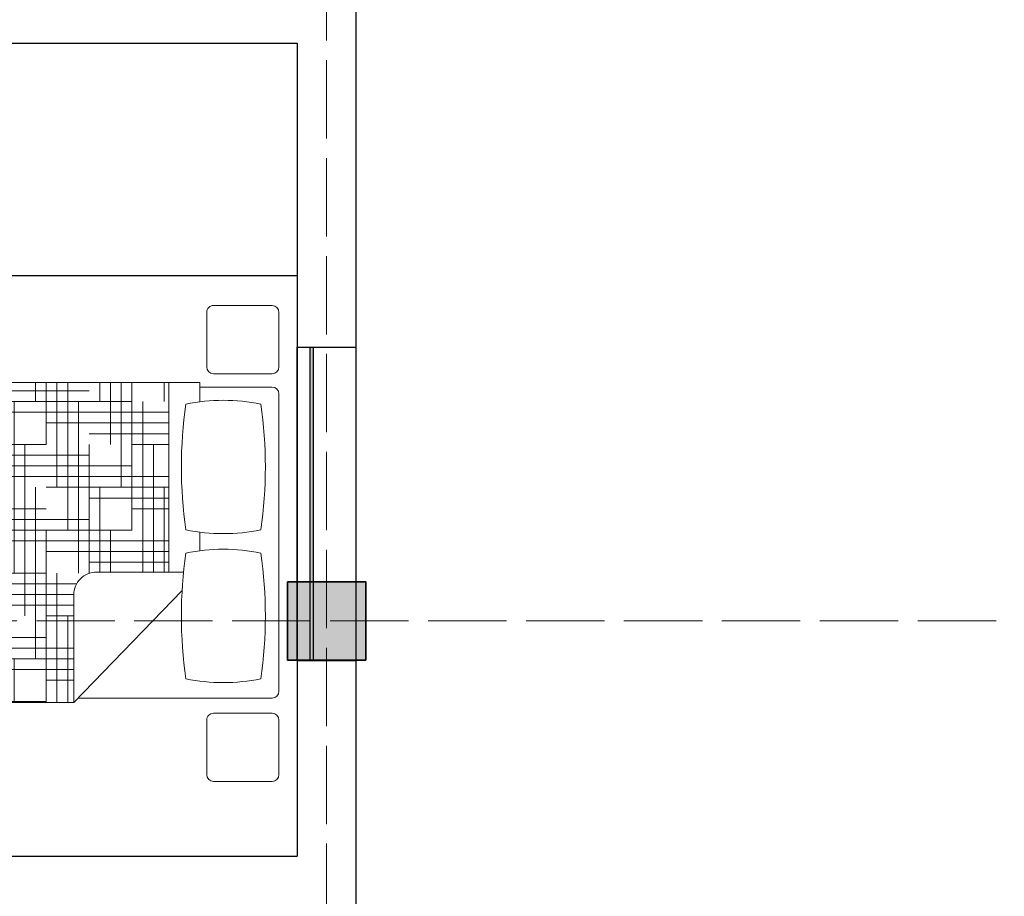
# Model space of a CAD drawing. Units: inches. Extents: x -113 to 5399, y -1393 to 3302.
# Tile 39 of 40: x 3612 to 3763, y 2903 to 3038. Entities that reach past the tile are written whole.
import ezdxf

# ---------------------------------------------------------------- set-up
doc = ezdxf.new("R2010")
doc.units = ezdxf.units.IN
doc.header["$MEASUREMENT"] = 0
doc.linetypes.add('ACAD_ISO02W100', pattern=[15, 12, -3])
for name, color, linetype, lineweight in [('A-ANNO-DIMS', 254, 'Continuous', 18), ('A-COLS', 7, 'Continuous', 35), ('furniture', 131, 'Continuous', 18), ('GRIDS', 7, 'ACAD_ISO02W100', 13), ('walls', 1, 'Continuous', 25), ('windows', 3, 'Continuous', 25)]:
    doc.layers.add(name, color=color, linetype=linetype, lineweight=lineweight)
doc.styles.get("Standard").update_dxf_attribs({"font": 'arial.ttf'})
doc.dimstyles.get("Standard").update_dxf_attribs({"dimtxt": 6, "dimasz": 0.18, "dimexe": 0.18, "dimexo": 0.0625, "dimgap": 0.09, "dimtad": 0, "dimtih": 1, "dimtoh": 1, "dimdec": 1, "dimzin": 0, "dimdsep": 46, "dimlunit": 4, "dimtxsty": 'Standard', "dimblk": 'ARCHTICK', "dimcen": 0.09, "dimadec": 0, "dimazin": 0, "dimtfac": 1, "dimtdec": 1, "dimtofl": 0, "dimtmove": 0, "dimatfit": 3, "dimfxl": 1, "dimtolj": 1, "dimtzin": 0, "dimarcsym": 0})

# ---------------------------------------------------------------- blocks, each defined once
blk = doc.blocks.new('*X4')
at = {"color": 0}
for p, q in [((4.3594, 18.5625), (4.3594, 18.6457)), ((4.5, 18), (4.5, 18.6457)), ((4.5469, 18.1875), (4.5469, 18.6457)), ((4.5938, 18.375), (4.5938, 18.6457)), ((4.6406, 18.5625), (4.6406, 18.6457)), ((4.7812, 18), (4.7812, 18.6457)), ((4.8281, 18.1875), (4.8281, 18.6457)), ((4.875, 18.375), (4.875, 18.6457)), ((4.9219, 18.5625), (4.9219, 18.6457)), ((5.0625, 18), (5.0625, 18.6457)), ((5.1094, 18.1875), (5.1094, 18.6457)), ((5.1562, 18.375), (5.1562, 18.6457)), ((5.2031, 18.5625), (5.2031, 18.6457)), ((5.3438, 18), (5.3438, 18.6457)), ((5.3906, 18.1875), (5.3906, 18.6457)), ((5.4375, 18.375), (5.4375, 18.6457)), ((5.4844, 18.5625), (5.4844, 18.6457)), ((4.6875, 18.6094), (5.4375, 18.6094)), ((5.625, 18), (5.625, 18.6287)), ((4.4531, 17.8169), (4.4531, 18.5625)), ((4.5, 18.5625), (5.25, 18.5625)), ((4.7344, 17.8125), (4.7344, 18.5625)), ((5.0156, 17.8125), (5.0156, 18.5625)), ((5.2969, 17.8125), (5.2969, 18.5625)), ((5.5781, 17.8125), (5.5781, 18.5625)), ((5.625, 18.5625), (5.6375, 18.5625)), ((4.3395, 18.5156), (5.0625, 18.5156)), ((5.4375, 18.5156), (5.6375, 18.5156)), ((4.3395, 18.4688), (4.875, 18.4688)), ((5.25, 18.4688), (5.6375, 18.4688)), ((4.3395, 18.4219), (4.6875, 18.4219)), ((5.0625, 18.4219), (5.6375, 18.4219)), ((4.3395, 18.375), (4.5, 18.375)), ((4.4062, 17.8169), (4.4062, 18.375)), ((4.6875, 17.8114), (4.6875, 18.375)), ((4.875, 18.375), (5.625, 18.375)), ((4.9688, 17.625), (4.9688, 18.375)), ((5.25, 17.625), (5.25, 18.375)), ((5.5312, 17.625), (5.5312, 18.375)), ((4.6875, 18.3281), (5.4375, 18.3281)), ((4.5, 18.2812), (5.25, 18.2812)), ((5.625, 18.2812), (5.6375, 18.2812)), ((4.3395, 18.2344), (5.0625, 18.2344)), ((5.4375, 18.2344), (5.6375, 18.2344)), ((4.3395, 18.1875), (4.875, 18.1875)), ((4.3594, 17.8169), (4.3594, 18.1875)), ((4.6406, 17.8169), (4.6406, 18.1875)), ((4.9219, 17.4375), (4.9219, 18.1875)), ((5.2031, 17.4375), (5.2031, 18.1875)), ((5.25, 18.1875), (5.6375, 18.1875)), ((5.4844, 17.4375), (5.4844, 18.1875)), ((4.3395, 18.1406), (4.6875, 18.1406)), ((5.0625, 18.1406), (5.6375, 18.1406)), ((4.3395, 18.0938), (4.5, 18.0938)), ((4.875, 18.0938), (5.625, 18.0938)), ((4.6875, 18.0469), (5.4375, 18.0469)), ((4.5, 18), (5.25, 18)), ((4.5938, 17.8169), (4.5938, 18)), ((4.875, 17.25), (4.875, 18)), ((5.1562, 17.25), (5.1562, 18)), ((5.4375, 17.25), (5.4375, 18)), ((5.625, 18), (5.6375, 18)), ((4.3395, 17.9531), (5.0625, 17.9531)), ((5.4375, 17.9531), (5.6375, 17.9531)), ((4.3395, 17.9062), (4.875, 17.9062)), ((5.25, 17.9062), (5.6375, 17.9062)), ((4.3395, 17.8594), (4.6875, 17.8594)), ((5.0625, 17.8594), (5.6375, 17.8594)), ((4.8281, 17.2457), (4.8281, 17.8125)), ((4.875, 17.8125), (5.625, 17.8125)), ((5.1094, 17.2457), (5.1094, 17.8125)), ((5.3906, 17.2457), (5.3906, 17.8125)), ((4.7421, 17.7656), (5.4375, 17.7656)), ((4.7548, 17.7188), (5.25, 17.7188)), ((5.625, 17.7188), (5.6375, 17.7188)), ((4.7548, 17.6719), (5.0625, 17.6719)), ((5.4375, 17.6719), (5.6375, 17.6719)), ((4.7548, 17.625), (4.875, 17.625)), ((4.7812, 17.2457), (4.7812, 17.625)), ((5.0625, 17.2457), (5.0625, 17.625)), ((5.25, 17.625), (5.6375, 17.625)), ((5.3438, 17.2457), (5.3438, 17.625)), ((5.625, 17.2627), (5.625, 17.625)), ((5.0625, 17.5781), (5.6375, 17.5781)), ((4.875, 17.5312), (5.625, 17.5312)), ((4.7548, 17.4844), (5.4375, 17.4844)), ((4.7548, 17.4375), (5.25, 17.4375)), ((5.0156, 17.2457), (5.0156, 17.4375)), ((5.2969, 17.2457), (5.2969, 17.4375)), ((5.5781, 17.2457), (5.5781, 17.4375)), ((5.625, 17.4375), (5.6375, 17.4375)), ((4.7548, 17.3906), (5.0625, 17.3906)), ((5.4375, 17.3906), (5.6375, 17.3906)), ((4.7548, 17.3438), (4.875, 17.3438)), ((5.25, 17.3438), (5.6375, 17.3438)), ((5.0625, 17.2969), (5.6375, 17.2969)), ((4.875, 17.25), (5.6077, 17.25)), ((4.9688, 17.2457), (4.9688, 17.25)), ((5.25, 17.2457), (5.25, 17.25)), ((5.5312, 17.2457), (5.5312, 17.25))]:
    blk.add_line(p, q, dxfattribs=at)
blk = doc.blocks.new('MAT-P01')
for p, q in [((0.0087, 0.8464), (0.2471, 0.8464)), ((0.3737, 0.8464), (1.6737, 0.8464)), ((1.7922, 0.8464), (2.0306, 0.8464)), ((-0.0213, 0.8164), (-0.0213, 0.5605)), ((0.2771, 0.8164), (0.2771, 0.5605)), ((0.3437, 0.8164), (0.3437, -0.0316)), ((1.7037, 0.8164), (1.7037, 0.5005)), ((1.7622, 0.8164), (1.7622, 0.5605)), ((2.0606, 0.8164), (2.0606, 0.5605)), ((0.0087, 0.5305), (0.2471, 0.5305)), ((1.7922, 0.5305), (2.0306, 0.5305)), ((0.9879, 0.5005), (1.0693, 0.5005)), ((1.6393, 0.5005), (1.7237, 0.5005)), ((1.7237, 0.5005), (1.7237, -0.8836)), ((0.8146, 0.423), (0.3237, -0.0509)), ((0.8949, 0.4293), (0.8949, 0.0491)), ((0.8949, 0.3643), (1.7237, 0.3643)), ((0.8949, 0.3643), (0.8949, 0.0491)), ((0.8949, 0.3643), (1.7237, 0.3643)), ((1.7237, 0.3643), (1.7237, -0.8836)), ((0.3237, -0.0509), (0.7949, -0.0509)), ((0.3237, -0.0509), (0.3237, -0.8836)), ((0.3737, -0.9336), (1.6737, -0.9336))]:
    blk.add_line(p, q)
for centre, radius, start, end in [((0.0087, 0.8164), 0.03, 90, 180), ((0.2471, 0.8164), 0.03, 0, 90), ((0.3737, 0.8164), 0.03, 90, 180), ((1.6737, 0.8164), 0.03, 0, 90), ((1.7922, 0.8164), 0.03, 90, 180), ((2.0306, 0.8164), 0.03, 0, 90), ((0.7029, -1.1436), 1.9306, 81.8162, 98.1838), ((1.3543, -1.1436), 1.9306, 81.8162, 98.1838), ((1.2251, 0.6034), 0.8138, 168.373, 191.627), ((0.1806, 0.6034), 0.8138, 348.373, 11.627), ((1.8766, 0.6034), 0.8138, 168.373, 191.627), ((0.8321, 0.6034), 0.8138, 348.373, 11.627), ((0.0087, 0.5605), 0.03, 180, 270), ((0.2471, 0.5605), 0.03, 270, 0), ((1.7922, 0.5605), 0.03, 180, 270), ((2.0306, 0.5605), 0.03, 270, 0), ((0.7029, 2.3504), 1.9306, 261.8162, 278.1838), ((1.3543, 2.3504), 1.9306, 261.8162, 278.1838), ((0.7949, 0.0491), 0.1, 270, 0), ((0.3737, -0.8836), 0.05, 180, 270), ((1.6737, -0.8836), 0.05, 270, 0)]:
    blk.add_arc(centre, radius, start, end)
at = {"rotation": 270}
blk.add_blockref('*X4', (-16.9221, 4.7038), dxfattribs=at)
blk = doc.blocks.new('_ArchTick')
at = {"color": 0, "linetype": 'ByBlock', "const_width": 0.15}
blk.add_lwpolyline([(-0.5, -0.5), (0.5, 0.5)], dxfattribs=at)
blk = doc.blocks.new('*D149')
at = {"layer": 'A-ANNO-DIMS', "color": 0, "lineweight": -2, "transparency": 16777216}
for p, q in [((3522.55, 2998.44), (3522.55, 2998.25)), ((3522.55, 2998.43), (3583.65, 2998.43)), ((3654.55, 2998.43), (3593.45, 2998.43)), ((3654.55, 2998.44), (3654.55, 2998.25))]:
    blk.add_line(p, q, dxfattribs=at)
at = {"layer": 'Defpoints', "color": 0, "transparency": 16777216}
for p in [(3522.55, 2998.5), (3522.55, 2998.43), (3654.55, 2998.5)]:
    blk.add_point(p, dxfattribs=at)
at = {"layer": 'A-ANNO-DIMS', "color": 0, "lineweight": -2, "transparency": 16777216, "xscale": 0.18, "yscale": 0.18, "zscale": 0.18, "rotation": 180}
blk.add_blockref('_ArchTick', (3522.55, 2998.43), dxfattribs=at)
at = {"layer": 'A-ANNO-DIMS', "color": 0, "lineweight": -2, "transparency": 16777216, "xscale": 0.18, "yscale": 0.18, "zscale": 0.18}
blk.add_blockref('_ArchTick', (3654.55, 2998.43), dxfattribs=at)
at = {"layer": 'A-ANNO-DIMS', "color": 0, "transparency": 16777216, "insert": (3588.55, 2998.43), "char_height": 6, "attachment_point": 5}
blk.add_mtext("\\A1;11'", dxfattribs=at)
blk = doc.blocks.new('WIN-PLAN-48IN')
h = blk.add_hatch(color=256)
h.dxf.hatch_style = 1
h.paths.add_polyline_path([(48, 2.5), (0, 2.5), (0, 2), (48, 2)])
for p, q in [((0, 9), (48, 9)), ((0, 0), (0, 9)), ((48, 9), (48, 0)), ((48, 2.5), (0, 2.5)), ((48, 2), (0, 2)), ((48, 0), (0, 0))]:
    blk.add_line(p, q)
blk = doc.blocks.new('COLUMN-12IN-SQUARE')
h = blk.add_hatch(color=256)
h.dxf.hatch_style = 1
h.paths.add_polyline_path([(6, 6), (-6, 6), (-6, -6), (6, -6)])
blk.add_lwpolyline([(-6, 6), (6, 6), (6, -6), (-6, -6)], close=True)

msp = doc.modelspace()

# ---------------------------------------------------------------- linework, layer by layer
at = {"layer": 'GRIDS'}
for p, q in [((3659.05, 3271.46), (3659.05, 2498.02)), ((3104.61, 2945.56), (3762.86, 2945.56))]:
    msp.add_line(p, q, dxfattribs=at)
at = {"layer": 'walls'}
for p, q in [((3663.55, 3230.06), (3663.55, 2580.06)), ((3562.55, 3034.06), (3654.55, 3034.06)), ((3654.55, 3034.06), (3654.55, 2909.56)), ((3505.55, 2909.56), (3654.55, 2909.56))]:
    msp.add_line(p, q, dxfattribs=at)

# ---------------------------------------------------------------- block references
at = {"layer": 'A-COLS'}
msp.add_blockref('COLUMN-12IN-SQUARE', (3659.05, 2945.56), dxfattribs=at)
at = {"layer": 'furniture', "xscale": -35.02364872074636, "yscale": 35.02364872074636, "zscale": 35.02364872074636, "rotation": 270}
msp.add_blockref('MAT-P01', (3622.12, 2921.72), dxfattribs=at)
at = {"layer": 'windows', "rotation": 270.0000000000029}
msp.add_blockref('WIN-PLAN-48IN', (3654.55, 2987.48), dxfattribs=at)

# ---------------------------------------------------------------- dimensions: what is measured, and where the dimension line sits
at = {"layer": 'A-ANNO-DIMS'}
dim = msp.add_linear_dim(base=(3522.55, 2998.43), p1=(3654.55, 2998.5), p2=(3522.55, 2998.5), dimstyle='Standard', override={"dimclrd": 0, "dimclre": 0, "dimclrt": 0}, dxfattribs=at)
dim.commit()
dim.dimension.update_dxf_attribs({"geometry": '*D149', "text_midpoint": (3588.55, 2998.43)})

doc.saveas('drawing.dxf')
